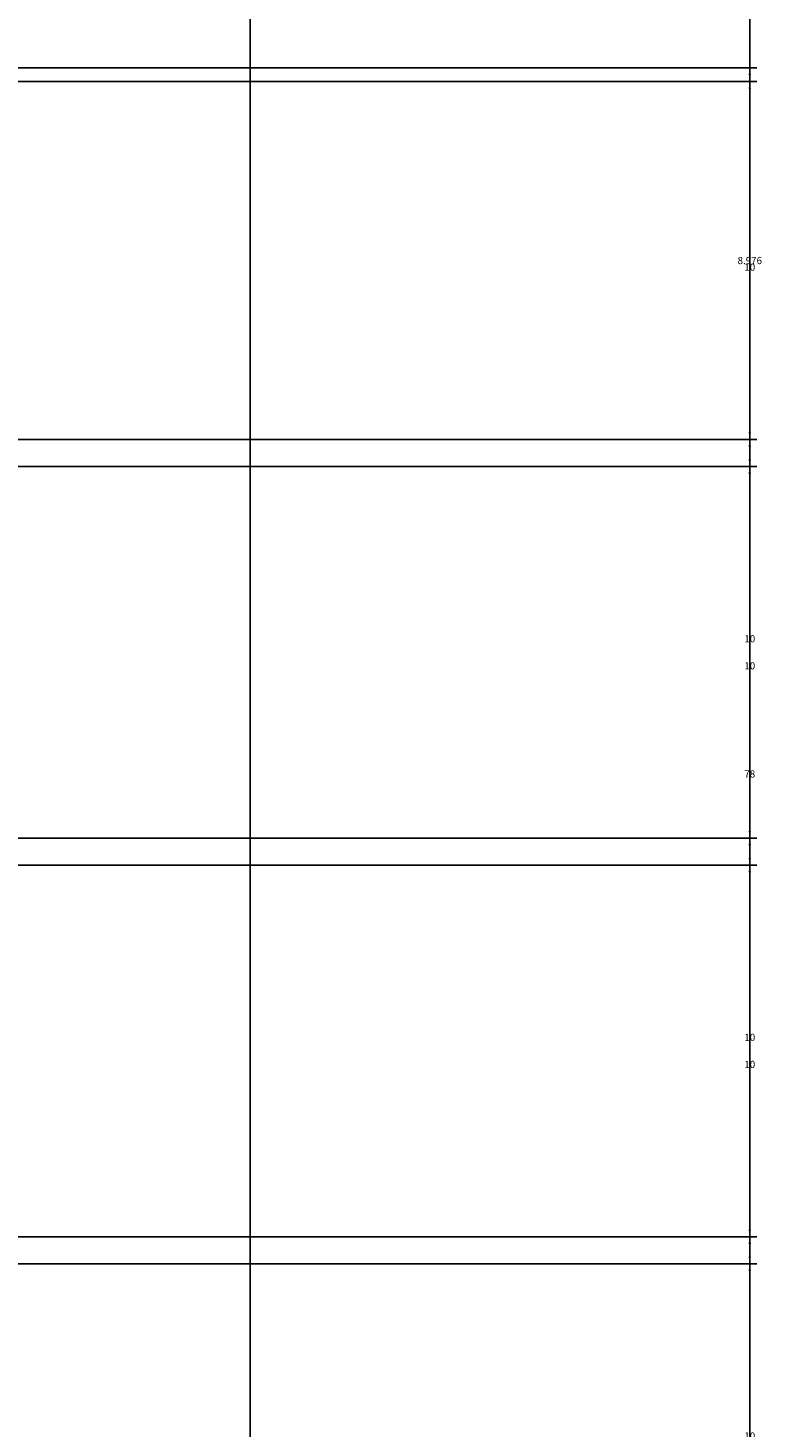
# Model space of a CAD drawing. Units: inches. Extents: x 2812 to 3051, y 1398 to 1659.
# Tile 37 of 65: x 3033 to 3051, y 1433 to 1468. Entities that reach past the tile are written whole.
import ezdxf

# ---------------------------------------------------------------- set-up
doc = ezdxf.new("R2010")
doc.units = ezdxf.units.IN
doc.layers.add('A-ANNO-DIMS', color=2, linetype='Continuous', lineweight=18)
doc.styles.get("Standard").update_dxf_attribs({"font": 'arial.ttf'})
doc.dimstyles.get("Standard").update_dxf_attribs({"dimtxt": 0.18, "dimasz": 0.18, "dimexe": 0.18, "dimexo": 0.0625, "dimgap": 0.09, "dimtad": 0, "dimtih": 1, "dimtoh": 1, "dimdec": 4, "dimzin": 0, "dimdsep": 46, "dimtxsty": 'Standard', "dimcen": 0.09, "dimadec": 0, "dimazin": 0, "dimtfac": 1, "dimtdec": 4, "dimtofl": 0, "dimtmove": 0, "dimatfit": 3, "dimfxl": 1, "dimtolj": 1, "dimtzin": 0, "dimarcsym": 0})

# ---------------------------------------------------------------- blocks, each defined once
blk = doc.blocks.new('*D34')
at = {"layer": 'A-ANNO-DIMS', "color": 0, "lineweight": -2, "transparency": 16777216}
for p, q in [((3038.462, 1593.482), (3038.462, 1397.505)), ((3027.385, 1550.757), (3027.385, 1397.505)), ((3027.565, 1397.685), (3032.468, 1397.685)), ((3038.282, 1397.685), (3033.379, 1397.685))]:
    blk.add_line(p, q, dxfattribs=at)
at = {"layer": 'A-ANNO-DIMS', "color": 0, "transparency": 16777216}
for points in [[(3027.565, 1397.715), (3027.565, 1397.655), (3027.385, 1397.685)], [(3038.282, 1397.715), (3038.282, 1397.655), (3038.462, 1397.685)]]:
    blk.add_solid(points, dxfattribs=at)
at = {"layer": 'Defpoints', "color": 0, "transparency": 16777216}
for p in [(3038.462, 1593.544), (3027.385, 1550.82), (3038.462, 1397.685)]:
    blk.add_point(p, dxfattribs=at)
at = {"layer": 'A-ANNO-DIMS', "color": 0, "transparency": 16777216, "insert": (3032.923, 1397.685), "char_height": 0.18, "attachment_point": 5}
blk.add_mtext('\\A1;11.077', dxfattribs=at)
blk = doc.blocks.new('*D48')
at = {"layer": 'A-ANNO-DIMS', "color": 0, "lineweight": -2, "transparency": 16777216}
for p, q in [((3006.385, 1487.973), (3006.385, 1397.505)), ((3036.385, 1409.973), (3036.385, 1397.505)), ((3006.565, 1397.685), (3021.166, 1397.685)), ((3036.205, 1397.685), (3021.603, 1397.685))]:
    blk.add_line(p, q, dxfattribs=at)
at = {"layer": 'A-ANNO-DIMS', "color": 0, "transparency": 16777216}
for points in [[(3006.565, 1397.715), (3006.565, 1397.655), (3006.385, 1397.685)], [(3036.205, 1397.715), (3036.205, 1397.655), (3036.385, 1397.685)]]:
    blk.add_solid(points, dxfattribs=at)
at = {"layer": 'Defpoints', "color": 0, "transparency": 16777216}
for p in [(3006.385, 1488.035), (3036.385, 1410.035), (3036.385, 1397.685)]:
    blk.add_point(p, dxfattribs=at)
at = {"layer": 'A-ANNO-DIMS', "color": 0, "transparency": 16777216, "insert": (3021.385, 1397.685), "char_height": 0.18, "attachment_point": 5}
blk.add_mtext('\\A1;30', dxfattribs=at)
blk = doc.blocks.new('*D54')
at = {"layer": 'A-ANNO-DIMS', "color": 0, "lineweight": -2, "transparency": 16777216}
for p, q in [((3036.447, 1488.035), (3051.178, 1488.035)), ((3050.998, 1487.855), (3050.998, 1449.217)), ((3050.998, 1410.215), (3050.998, 1448.853)), ((3036.447, 1410.035), (3051.178, 1410.035))]:
    blk.add_line(p, q, dxfattribs=at)
at = {"layer": 'A-ANNO-DIMS', "color": 0, "transparency": 16777216}
for points in [[(3050.968, 1487.855), (3051.028, 1487.855), (3050.998, 1488.035)], [(3050.968, 1410.215), (3051.028, 1410.215), (3050.998, 1410.035)]]:
    blk.add_solid(points, dxfattribs=at)
at = {"layer": 'Defpoints', "color": 0, "transparency": 16777216}
for p in [(3036.385, 1488.035), (3050.998, 1488.035), (3036.385, 1410.035)]:
    blk.add_point(p, dxfattribs=at)
at = {"layer": 'A-ANNO-DIMS', "color": 0, "transparency": 16777216, "insert": (3050.998, 1449.035), "char_height": 0.18, "attachment_point": 5}
blk.add_mtext('\\A1;78', dxfattribs=at)
blk = doc.blocks.new('*D65')
at = {"layer": 'A-ANNO-DIMS', "color": 0, "lineweight": -2, "transparency": 16777216}
for p, q in [((2920.62, 1437.426), (3051.178, 1437.426)), ((3050.998, 1437.246), (3050.998, 1432.608)), ((3050.998, 1427.606), (3050.998, 1432.245)), ((2929.438, 1427.426), (3051.178, 1427.426))]:
    blk.add_line(p, q, dxfattribs=at)
at = {"layer": 'A-ANNO-DIMS', "color": 0, "transparency": 16777216}
for points in [[(3050.968, 1437.246), (3051.028, 1437.246), (3050.998, 1437.426)], [(3050.968, 1427.606), (3051.028, 1427.606), (3050.998, 1427.426)]]:
    blk.add_solid(points, dxfattribs=at)
at = {"layer": 'Defpoints', "color": 0, "transparency": 16777216}
for p in [(2920.558, 1437.426), (3050.998, 1437.426), (2929.375, 1427.426)]:
    blk.add_point(p, dxfattribs=at)
at = {"layer": 'A-ANNO-DIMS', "color": 0, "transparency": 16777216, "insert": (3050.998, 1432.426), "char_height": 0.18, "attachment_point": 5}
blk.add_mtext('\\A1;10', dxfattribs=at)
blk = doc.blocks.new('*D66')
at = {"layer": 'A-ANNO-DIMS', "color": 0, "lineweight": -2, "transparency": 16777216}
for p, q in [((2914.018, 1447.426), (3051.178, 1447.426)), ((3050.998, 1447.246), (3050.998, 1442.608)), ((3050.998, 1437.606), (3050.998, 1442.245)), ((2920.62, 1437.426), (3051.178, 1437.426))]:
    blk.add_line(p, q, dxfattribs=at)
at = {"layer": 'A-ANNO-DIMS', "color": 0, "transparency": 16777216}
for points in [[(3050.968, 1447.246), (3051.028, 1447.246), (3050.998, 1447.426)], [(3050.968, 1437.606), (3051.028, 1437.606), (3050.998, 1437.426)]]:
    blk.add_solid(points, dxfattribs=at)
at = {"layer": 'Defpoints', "color": 0, "transparency": 16777216}
for p in [(2913.955, 1447.426), (3050.998, 1447.426), (2920.558, 1437.426)]:
    blk.add_point(p, dxfattribs=at)
at = {"layer": 'A-ANNO-DIMS', "color": 0, "transparency": 16777216, "insert": (3050.998, 1442.426), "char_height": 0.18, "attachment_point": 5}
blk.add_mtext('\\A1;10', dxfattribs=at)
blk = doc.blocks.new('*D67')
at = {"layer": 'A-ANNO-DIMS', "color": 0, "lineweight": -2, "transparency": 16777216}
for p, q in [((2906.065, 1457.426), (3051.178, 1457.426)), ((3050.998, 1457.246), (3050.998, 1452.608)), ((3050.998, 1447.606), (3050.998, 1452.245)), ((2914.018, 1447.426), (3051.178, 1447.426))]:
    blk.add_line(p, q, dxfattribs=at)
at = {"layer": 'A-ANNO-DIMS', "color": 0, "transparency": 16777216}
for points in [[(3050.968, 1457.246), (3051.028, 1457.246), (3050.998, 1457.426)], [(3050.968, 1447.606), (3051.028, 1447.606), (3050.998, 1447.426)]]:
    blk.add_solid(points, dxfattribs=at)
at = {"layer": 'Defpoints', "color": 0, "transparency": 16777216}
for p in [(2906.002, 1457.426), (3050.998, 1457.426), (2913.955, 1447.426)]:
    blk.add_point(p, dxfattribs=at)
at = {"layer": 'A-ANNO-DIMS', "color": 0, "transparency": 16777216, "insert": (3050.998, 1452.426), "char_height": 0.18, "attachment_point": 5}
blk.add_mtext('\\A1;10', dxfattribs=at)
blk = doc.blocks.new('*D68')
at = {"layer": 'A-ANNO-DIMS', "color": 0, "lineweight": -2, "transparency": 16777216}
for p, q in [((2898.12, 1466.402), (3051.178, 1466.402)), ((3050.998, 1466.222), (3050.998, 1462.096)), ((3050.998, 1457.606), (3050.998, 1461.733)), ((2906.065, 1457.426), (3051.178, 1457.426))]:
    blk.add_line(p, q, dxfattribs=at)
at = {"layer": 'A-ANNO-DIMS', "color": 0, "transparency": 16777216}
for points in [[(3050.968, 1466.222), (3051.028, 1466.222), (3050.998, 1466.402)], [(3050.968, 1457.606), (3051.028, 1457.606), (3050.998, 1457.426)]]:
    blk.add_solid(points, dxfattribs=at)
at = {"layer": 'Defpoints', "color": 0, "transparency": 16777216}
for p in [(2898.058, 1466.402), (3050.998, 1466.402), (2906.002, 1457.426)]:
    blk.add_point(p, dxfattribs=at)
at = {"layer": 'A-ANNO-DIMS', "color": 0, "transparency": 16777216, "insert": (3050.998, 1461.914), "char_height": 0.18, "attachment_point": 5}
blk.add_mtext('\\A1;8.976', dxfattribs=at)
blk = doc.blocks.new('*D79')
at = {"layer": 'A-ANNO-DIMS', "color": 0, "lineweight": -2, "transparency": 16777216}
for p, q in [((3003.284, 1436.747), (3051.178, 1436.747)), ((3050.998, 1436.567), (3050.998, 1431.929)), ((3050.998, 1426.927), (3050.998, 1431.565)), ((3012.899, 1426.747), (3051.178, 1426.747))]:
    blk.add_line(p, q, dxfattribs=at)
at = {"layer": 'A-ANNO-DIMS', "color": 0, "transparency": 16777216}
for points in [[(3050.968, 1436.567), (3051.028, 1436.567), (3050.998, 1436.747)], [(3050.968, 1426.927), (3051.028, 1426.927), (3050.998, 1426.747)]]:
    blk.add_solid(points, dxfattribs=at)
at = {"layer": 'Defpoints', "color": 0, "transparency": 16777216}
for p in [(3003.221, 1436.747), (3050.998, 1436.747), (3012.837, 1426.747)]:
    blk.add_point(p, dxfattribs=at)
at = {"layer": 'A-ANNO-DIMS', "color": 0, "transparency": 16777216, "insert": (3050.998, 1431.747), "char_height": 0.18, "attachment_point": 5}
blk.add_mtext('\\A1;10', dxfattribs=at)
blk = doc.blocks.new('*D80')
at = {"layer": 'A-ANNO-DIMS', "color": 0, "lineweight": -2, "transparency": 16777216}
for p, q in [((2996.018, 1446.747), (3051.178, 1446.747)), ((3050.998, 1446.567), (3050.998, 1441.929)), ((3050.998, 1436.927), (3050.998, 1441.565)), ((3003.284, 1436.747), (3051.178, 1436.747))]:
    blk.add_line(p, q, dxfattribs=at)
at = {"layer": 'A-ANNO-DIMS', "color": 0, "transparency": 16777216}
for points in [[(3050.968, 1446.567), (3051.028, 1446.567), (3050.998, 1446.747)], [(3050.968, 1436.927), (3051.028, 1436.927), (3050.998, 1436.747)]]:
    blk.add_solid(points, dxfattribs=at)
at = {"layer": 'Defpoints', "color": 0, "transparency": 16777216}
for p in [(2995.956, 1446.747), (3050.998, 1446.747), (3003.221, 1436.747)]:
    blk.add_point(p, dxfattribs=at)
at = {"layer": 'A-ANNO-DIMS', "color": 0, "transparency": 16777216, "insert": (3050.998, 1441.747), "char_height": 0.18, "attachment_point": 5}
blk.add_mtext('\\A1;10', dxfattribs=at)
blk = doc.blocks.new('*D81')
at = {"layer": 'A-ANNO-DIMS', "color": 0, "lineweight": -2, "transparency": 16777216}
for p, q in [((2988.31, 1456.747), (3051.178, 1456.747)), ((3050.998, 1456.567), (3050.998, 1451.929)), ((3050.998, 1446.927), (3050.998, 1451.565)), ((2996.018, 1446.747), (3051.178, 1446.747))]:
    blk.add_line(p, q, dxfattribs=at)
at = {"layer": 'A-ANNO-DIMS', "color": 0, "transparency": 16777216}
for points in [[(3050.968, 1456.567), (3051.028, 1456.567), (3050.998, 1456.747)], [(3050.968, 1446.927), (3051.028, 1446.927), (3050.998, 1446.747)]]:
    blk.add_solid(points, dxfattribs=at)
at = {"layer": 'Defpoints', "color": 0, "transparency": 16777216}
for p in [(2988.248, 1456.747), (3050.998, 1456.747), (2995.956, 1446.747)]:
    blk.add_point(p, dxfattribs=at)
at = {"layer": 'A-ANNO-DIMS', "color": 0, "transparency": 16777216, "insert": (3050.998, 1451.747), "char_height": 0.18, "attachment_point": 5}
blk.add_mtext('\\A1;10', dxfattribs=at)
blk = doc.blocks.new('*D82')
at = {"layer": 'A-ANNO-DIMS', "color": 0, "lineweight": -2, "transparency": 16777216}
for p, q in [((2978.018, 1466.747), (3051.178, 1466.747)), ((3050.998, 1466.567), (3050.998, 1461.929)), ((3050.998, 1456.927), (3050.998, 1461.565)), ((2988.31, 1456.747), (3051.178, 1456.747))]:
    blk.add_line(p, q, dxfattribs=at)
at = {"layer": 'A-ANNO-DIMS', "color": 0, "transparency": 16777216}
for points in [[(3050.968, 1466.567), (3051.028, 1466.567), (3050.998, 1466.747)], [(3050.968, 1456.927), (3051.028, 1456.927), (3050.998, 1456.747)]]:
    blk.add_solid(points, dxfattribs=at)
at = {"layer": 'Defpoints', "color": 0, "transparency": 16777216}
for p in [(2977.956, 1466.747), (3050.998, 1466.747), (2988.248, 1456.747)]:
    blk.add_point(p, dxfattribs=at)
at = {"layer": 'A-ANNO-DIMS', "color": 0, "transparency": 16777216, "insert": (3050.998, 1461.747), "char_height": 0.18, "attachment_point": 5}
blk.add_mtext('\\A1;10', dxfattribs=at)

msp = doc.modelspace()

# ---------------------------------------------------------------- dimensions: what is measured, and where the dimension line sits
at = {"layer": 'A-ANNO-DIMS'}
for base, p1, p2, override, picture, middle in [((3038.4621, 1397.6854), (3027.3849, 1550.82), (3038.4621, 1593.5441), {"dimdec": 3, "dimlfac": 1, "dimrnd": 0, "dimzin": 0, "dimdsep": 46, "dimlunit": 2}, '*D34', (3032.9235, 1397.6854)), ((3036.3849, 1397.6854), (3006.3849, 1488.0354), (3036.3849, 1410.0354), {"dimdec": 0, "dimlfac": 1, "dimrnd": 0, "dimzin": 0, "dimdsep": 46, "dimlunit": 2}, '*D48', (3021.3849, 1397.6854))]:
    dim = msp.add_linear_dim(base=base, p1=p1, p2=p2, dimstyle='Standard', override=override, dxfattribs=at)
    dim.commit()
    dim.dimension.update_dxf_attribs({"geometry": picture, "text_midpoint": middle})
for base, p1, p2, override, picture, middle in [((3050.998, 1488.0354), (3036.3849, 1410.0354), (3036.3849, 1488.0354), {"dimdec": 0, "dimlfac": 1, "dimrnd": 0, "dimzin": 0, "dimdsep": 46, "dimlunit": 2}, '*D54', (3050.998, 1449.0354)), ((3050.998, 1466.7474), (2988.2478, 1456.7474), (2977.9558, 1466.7474), {"dimdec": 0, "dimlfac": 1, "dimrnd": 0, "dimzin": 0, "dimdsep": 46, "dimlunit": 2}, '*D82', (3050.998, 1461.7474)), ((3050.998, 1466.4024), (2906.0021, 1457.4265), (2898.0577, 1466.4024), {"dimdec": 3, "dimlfac": 1, "dimrnd": 0, "dimzin": 0, "dimdsep": 46, "dimlunit": 2}, '*D68', (3050.998, 1461.9144)), ((3050.998, 1457.4265), (2913.9551, 1447.4265), (2906.0021, 1457.4265), {"dimdec": 0, "dimlfac": 1, "dimrnd": 0, "dimzin": 0, "dimdsep": 46, "dimlunit": 2}, '*D67', (3050.998, 1452.4265)), ((3050.998, 1456.7474), (2995.9558, 1446.7474), (2988.2478, 1456.7474), {"dimdec": 0, "dimlfac": 1, "dimrnd": 0, "dimzin": 0, "dimdsep": 46, "dimlunit": 2}, '*D81', (3050.998, 1451.7474)), ((3050.998, 1447.4265), (2920.5577, 1437.4265), (2913.9551, 1447.4265), {"dimdec": 0, "dimlfac": 1, "dimrnd": 0, "dimzin": 0, "dimdsep": 46, "dimlunit": 2}, '*D66', (3050.998, 1442.4265)), ((3050.998, 1446.7474), (3003.2213, 1436.7474), (2995.9558, 1446.7474), {"dimdec": 0, "dimlfac": 1, "dimrnd": 0, "dimzin": 0, "dimdsep": 46, "dimlunit": 2}, '*D80', (3050.998, 1441.7474)), ((3050.998, 1437.4265), (2929.3751, 1427.4265), (2920.5577, 1437.4265), {"dimdec": 0, "dimlfac": 1, "dimrnd": 0, "dimzin": 0, "dimdsep": 46, "dimlunit": 2}, '*D65', (3050.998, 1432.4265)), ((3050.998, 1436.7474), (3012.8368, 1426.7474), (3003.2213, 1436.7474), {"dimdec": 0, "dimlfac": 1, "dimrnd": 0, "dimzin": 0, "dimdsep": 46, "dimlunit": 2}, '*D79', (3050.998, 1431.7474))]:
    dim = msp.add_linear_dim(base=base, p1=p1, p2=p2, angle=90, dimstyle='Standard', override=override, dxfattribs=at)
    dim.commit()
    dim.dimension.update_dxf_attribs({"geometry": picture, "text_midpoint": middle})

doc.saveas('drawing.dxf')
